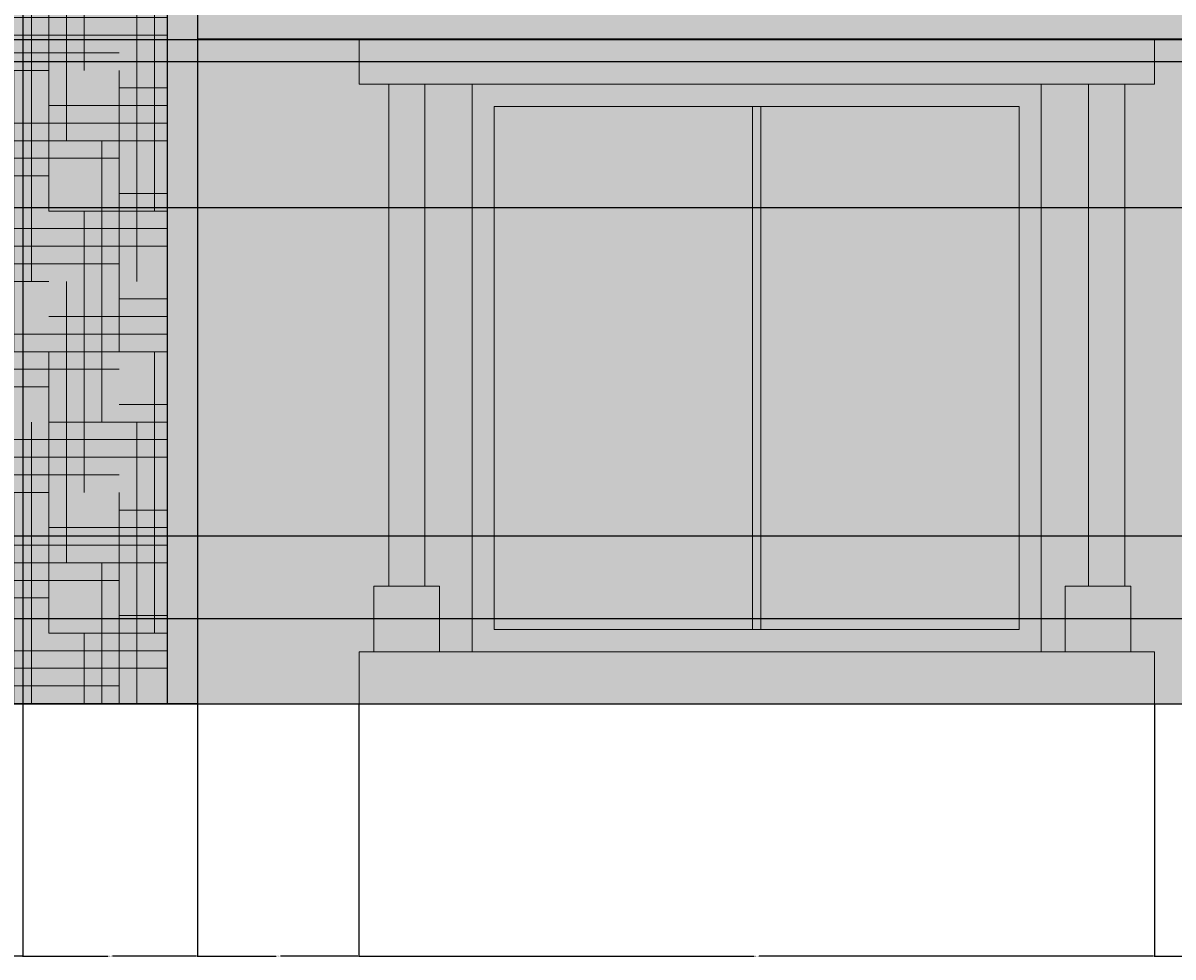
# Model space of a CAD drawing. Units: inches. Extents: x 3024 to 4744, y 1110 to 2100.
# Tile 14 of 29: x 3450 to 3657, y 1110 to 1279. Entities that reach past the tile are written whole.
import ezdxf

# ---------------------------------------------------------------- set-up
doc = ezdxf.new("R2010")
doc.units = ezdxf.units.IN
for name, color, linetype, lineweight in [('A-ANNO-DIMS', 2, 'Continuous', 18), ('A-ELEV', 7, 'Continuous', 25), ('A-ELEV-PATT', 252, 'Continuous', 13), ('A-GLAZ', 4, 'Continuous', 18)]:
    doc.layers.add(name, color=color, linetype=linetype, lineweight=lineweight)
doc.styles.get("Standard").update_dxf_attribs({"font": 'arial.ttf'})
doc.dimstyles.get("Standard").update_dxf_attribs({"dimtxt": 0.18, "dimasz": 0.18, "dimexe": 0.18, "dimexo": 0.0625, "dimgap": 0.09, "dimtad": 0, "dimtih": 1, "dimtoh": 1, "dimdec": 1, "dimzin": 0, "dimdsep": 46, "dimlunit": 3, "dimtxsty": 'Standard', "dimcen": 0.09, "dimadec": 0, "dimazin": 0, "dimtfac": 1, "dimtdec": 1, "dimtofl": 0, "dimtmove": 0, "dimatfit": 3, "dimfxl": 1, "dimtolj": 1, "dimtzin": 0, "dimarcsym": 0})

# ---------------------------------------------------------------- blocks, each defined once
blk = doc.blocks.new('WIN-BALCONY-A')
for p, q in [((3169.4, 1897.49), (3148.97, 1897.49)), ((3169.4, 1897.49), (3148.97, 1897.49)), ((3169.4, 1897.49), (3292.61, 1897.49)), ((3169.4, 1897.49), (3292.61, 1897.49)), ((3169.4, 1795.04), (3148.97, 1795.04)), ((3169.4, 1795.04), (3148.97, 1795.04)), ((3169.4, 1795.04), (3292.61, 1795.04)), ((3169.4, 1795.04), (3292.61, 1795.04))]:
    blk.add_line(p, q)
for points in [[(3148.97, 1897.49), (3148.97, 1905.61), (3292.61, 1905.61), (3292.61, 1897.49)], [(3148.97, 1897.49), (3148.97, 1905.61), (3292.61, 1905.61), (3292.61, 1897.49)], [(3292.61, 1795.04), (3292.61, 1785.61), (3148.97, 1785.61), (3148.97, 1795.04)], [(3292.61, 1795.04), (3292.61, 1785.61), (3148.97, 1785.61), (3148.97, 1795.04)]]:
    blk.add_lwpolyline(points)
for points in [[(3154.33, 1806.87), (3160.86, 1806.87), (3160.86, 1897.49), (3154.33, 1897.49)], [(3154.33, 1806.87), (3160.86, 1806.87), (3160.86, 1897.49), (3154.33, 1897.49)], [(3272.18, 1795.04), (3169.4, 1795.04), (3169.4, 1897.49), (3272.18, 1897.49)], [(3272.18, 1795.04), (3169.4, 1795.04), (3169.4, 1897.49), (3272.18, 1897.49)], [(3287.25, 1806.87), (3280.72, 1806.87), (3280.72, 1897.49), (3287.25, 1897.49)], [(3287.25, 1806.87), (3280.72, 1806.87), (3280.72, 1897.49), (3287.25, 1897.49)], [(3268.18, 1799.04), (3173.4, 1799.04), (3173.4, 1893.49), (3268.18, 1893.49)], [(3268.18, 1799.04), (3173.4, 1799.04), (3173.4, 1893.49), (3268.18, 1893.49)], [(3220.05, 1893.49), (3221.52, 1893.49), (3221.52, 1799.04), (3220.05, 1799.04)], [(3220.05, 1893.49), (3221.52, 1893.49), (3221.52, 1799.04), (3220.05, 1799.04)], [(3163.53, 1795.04), (3151.66, 1795.04), (3151.66, 1806.87), (3163.53, 1806.87)], [(3163.53, 1795.04), (3151.66, 1795.04), (3151.66, 1806.87), (3163.53, 1806.87)], [(3276.51, 1795.04), (3288.38, 1795.04), (3288.38, 1806.87), (3276.51, 1806.87)], [(3276.51, 1795.04), (3288.38, 1795.04), (3288.38, 1806.87), (3276.51, 1806.87)]]:
    blk.add_lwpolyline(points, close=True)
blk = doc.blocks.new('*D57')
at = {"layer": 'A-ANNO-DIMS', "color": 0, "lineweight": -2, "transparency": 16777216}
for p, q in [((3361.22, 1329.46), (3361.22, 1109.93)), ((3449.72, 1329.46), (3449.72, 1109.93)), ((3361.4, 1110.11), (3405.15, 1110.11)), ((3449.54, 1110.11), (3405.8, 1110.11))]:
    blk.add_line(p, q, dxfattribs=at)
at = {"layer": 'A-ANNO-DIMS', "color": 0, "transparency": 16777216}
for points in [[(3361.4, 1110.14), (3361.4, 1110.08), (3361.22, 1110.11)], [(3449.54, 1110.14), (3449.54, 1110.08), (3449.72, 1110.11)]]:
    blk.add_solid(points, dxfattribs=at)
at = {"layer": 'Defpoints', "color": 0, "transparency": 16777216}
for p in [(3361.22, 1329.52), (3449.72, 1329.52), (3449.72, 1110.11)]:
    blk.add_point(p, dxfattribs=at)
at = {"layer": 'A-ANNO-DIMS', "color": 0, "transparency": 16777216, "insert": (3405.47, 1110.11), "char_height": 0.18, "attachment_point": 5}
blk.add_mtext('\\A1;88.5', dxfattribs=at)
blk = doc.blocks.new('*D58')
at = {"layer": 'A-ANNO-DIMS', "color": 0, "lineweight": -2, "transparency": 16777216}
for p, q in [((3449.72, 1329.46), (3449.72, 1109.93)), ((3481.24, 1155.55), (3481.24, 1109.93)), ((3449.9, 1110.11), (3465.09, 1110.11)), ((3481.06, 1110.11), (3465.87, 1110.11))]:
    blk.add_line(p, q, dxfattribs=at)
at = {"layer": 'A-ANNO-DIMS', "color": 0, "transparency": 16777216}
for points in [[(3449.9, 1110.14), (3449.9, 1110.08), (3449.72, 1110.11)], [(3481.06, 1110.14), (3481.06, 1110.08), (3481.24, 1110.11)]]:
    blk.add_solid(points, dxfattribs=at)
at = {"layer": 'Defpoints', "color": 0, "transparency": 16777216}
for p in [(3449.72, 1329.52), (3481.24, 1155.61), (3481.24, 1110.11)]:
    blk.add_point(p, dxfattribs=at)
at = {"layer": 'A-ANNO-DIMS', "color": 0, "transparency": 16777216, "insert": (3465.48, 1110.11), "char_height": 0.18, "attachment_point": 5}
blk.add_mtext('\\A1;31.52', dxfattribs=at)
blk = doc.blocks.new('*D59')
at = {"layer": 'A-ANNO-DIMS', "color": 0, "lineweight": -2, "transparency": 16777216}
for p, q in [((3481.24, 1155.55), (3481.24, 1109.93)), ((3510.4, 1155.55), (3510.4, 1109.93)), ((3481.42, 1110.11), (3495.43, 1110.11)), ((3510.22, 1110.11), (3496.22, 1110.11))]:
    blk.add_line(p, q, dxfattribs=at)
at = {"layer": 'A-ANNO-DIMS', "color": 0, "transparency": 16777216}
for points in [[(3481.42, 1110.14), (3481.42, 1110.08), (3481.24, 1110.11)], [(3510.22, 1110.14), (3510.22, 1110.08), (3510.4, 1110.11)]]:
    blk.add_solid(points, dxfattribs=at)
at = {"layer": 'Defpoints', "color": 0, "transparency": 16777216}
for p in [(3481.24, 1155.61), (3510.4, 1155.61), (3510.4, 1110.11)]:
    blk.add_point(p, dxfattribs=at)
at = {"layer": 'A-ANNO-DIMS', "color": 0, "transparency": 16777216, "insert": (3495.82, 1110.11), "char_height": 0.18, "attachment_point": 5}
blk.add_mtext('\\A1;29.16', dxfattribs=at)
blk = doc.blocks.new('*D60')
at = {"layer": 'A-ANNO-DIMS', "color": 0, "lineweight": -2, "transparency": 16777216}
for p, q in [((3510.4, 1155.55), (3510.4, 1109.93)), ((3654.04, 1155.55), (3654.04, 1109.93)), ((3510.58, 1110.11), (3581.76, 1110.11)), ((3653.86, 1110.11), (3582.67, 1110.11))]:
    blk.add_line(p, q, dxfattribs=at)
at = {"layer": 'A-ANNO-DIMS', "color": 0, "transparency": 16777216}
for points in [[(3510.58, 1110.14), (3510.58, 1110.08), (3510.4, 1110.11)], [(3653.86, 1110.14), (3653.86, 1110.08), (3654.04, 1110.11)]]:
    blk.add_solid(points, dxfattribs=at)
at = {"layer": 'Defpoints', "color": 0, "transparency": 16777216}
for p in [(3510.4, 1155.61), (3654.04, 1155.61), (3654.04, 1110.11)]:
    blk.add_point(p, dxfattribs=at)
at = {"layer": 'A-ANNO-DIMS', "color": 0, "transparency": 16777216, "insert": (3582.22, 1110.11), "char_height": 0.18, "attachment_point": 5}
blk.add_mtext('\\A1;143.64', dxfattribs=at)
blk = doc.blocks.new('*D61')
at = {"layer": 'A-ANNO-DIMS', "color": 0, "lineweight": -2, "transparency": 16777216}
for p, q in [((3654.04, 1155.55), (3654.04, 1109.93)), ((3688.56, 1155.55), (3688.56, 1109.93)), ((3654.22, 1110.11), (3670.91, 1110.11)), ((3688.38, 1110.11), (3671.69, 1110.11))]:
    blk.add_line(p, q, dxfattribs=at)
at = {"layer": 'A-ANNO-DIMS', "color": 0, "transparency": 16777216}
for points in [[(3654.22, 1110.14), (3654.22, 1110.08), (3654.04, 1110.11)], [(3688.38, 1110.14), (3688.38, 1110.08), (3688.56, 1110.11)]]:
    blk.add_solid(points, dxfattribs=at)
at = {"layer": 'Defpoints', "color": 0, "transparency": 16777216}
for p in [(3654.04, 1155.61), (3688.56, 1155.61), (3688.56, 1110.11)]:
    blk.add_point(p, dxfattribs=at)
at = {"layer": 'A-ANNO-DIMS', "color": 0, "transparency": 16777216, "insert": (3671.3, 1110.11), "char_height": 0.18, "attachment_point": 5}
blk.add_mtext('\\A1;34.52', dxfattribs=at)
blk = doc.blocks.new('*D64')
at = {"layer": 'A-ANNO-DIMS', "color": 0, "lineweight": -2, "transparency": 16777216}
for p, q in [((3069.79, 1241.5), (3069.79, 2100.44)), ((3069.97, 2100.26), (3405.08, 2100.26)), ((3740.97, 2100.26), (3405.87, 2100.26)), ((3741.15, 1241.5), (3741.15, 2100.44))]:
    blk.add_line(p, q, dxfattribs=at)
at = {"layer": 'A-ANNO-DIMS', "color": 0, "transparency": 16777216}
for points in [[(3069.97, 2100.29), (3069.97, 2100.23), (3069.79, 2100.26)], [(3740.97, 2100.29), (3740.97, 2100.23), (3741.15, 2100.26)]]:
    blk.add_solid(points, dxfattribs=at)
at = {"layer": 'Defpoints', "color": 0, "transparency": 16777216}
for p in [(3741.15, 2100.26), (3069.79, 1241.43), (3741.15, 1241.43)]:
    blk.add_point(p, dxfattribs=at)
at = {"layer": 'A-ANNO-DIMS', "color": 0, "transparency": 16777216, "insert": (3405.47, 2100.26), "char_height": 0.18, "attachment_point": 5}
blk.add_mtext('\\A1;671.4', dxfattribs=at)
blk = doc.blocks.new('*D75')
at = {"layer": 'A-ANNO-DIMS', "color": 0, "lineweight": -2, "transparency": 16777216}
for p, q in [((3491.89, 2054.76), (3786.83, 2054.76)), ((3786.65, 2054.58), (3786.65, 1605.37)), ((3786.65, 1155.79), (3786.65, 1605)), ((3741.21, 1155.61), (3786.83, 1155.61))]:
    blk.add_line(p, q, dxfattribs=at)
at = {"layer": 'A-ANNO-DIMS', "color": 0, "transparency": 16777216}
for points in [[(3786.62, 2054.58), (3786.68, 2054.58), (3786.65, 2054.76)], [(3786.62, 1155.79), (3786.68, 1155.79), (3786.65, 1155.61)]]:
    blk.add_solid(points, dxfattribs=at)
at = {"layer": 'Defpoints', "color": 0, "transparency": 16777216}
for p in [(3491.83, 2054.76), (3786.65, 2054.76), (3741.15, 1155.61)]:
    blk.add_point(p, dxfattribs=at)
at = {"layer": 'A-ANNO-DIMS', "color": 0, "transparency": 16777216, "insert": (3786.65, 1605.18), "char_height": 0.18, "attachment_point": 5}
blk.add_mtext('\\A1;899.1', dxfattribs=at)
blk = doc.blocks.new('*D120')
at = {"layer": 'A-ANNO-DIMS', "color": 0, "lineweight": -2, "transparency": 16777216}
for p, q in [((3270.45, 1271.61), (3786.83, 1271.61)), ((3786.65, 1271.43), (3786.65, 1221.5)), ((3786.65, 1171.2), (3786.65, 1221.14)), ((3274.45, 1171.02), (3786.83, 1171.02))]:
    blk.add_line(p, q, dxfattribs=at)
at = {"layer": 'A-ANNO-DIMS', "color": 0, "transparency": 16777216}
for points in [[(3786.62, 1271.43), (3786.68, 1271.43), (3786.65, 1271.61)], [(3786.62, 1171.2), (3786.68, 1171.2), (3786.65, 1171.02)]]:
    blk.add_solid(points, dxfattribs=at)
at = {"layer": 'Defpoints', "color": 0, "transparency": 16777216}
for p in [(3270.39, 1271.61), (3786.65, 1271.61), (3274.39, 1171.02)]:
    blk.add_point(p, dxfattribs=at)
at = {"layer": 'A-ANNO-DIMS', "color": 0, "transparency": 16777216, "insert": (3786.65, 1221.32), "char_height": 0.18, "attachment_point": 5}
blk.add_mtext('\\A1;100.59', dxfattribs=at)
blk = doc.blocks.new('*D121')
at = {"layer": 'A-ANNO-DIMS', "color": 0, "lineweight": -2, "transparency": 16777216}
for p, q in [((3274.45, 1275.61), (3786.83, 1275.61)), ((3786.65, 1275.43), (3786.65, 1273.79)), ((3786.65, 1271.79), (3786.65, 1273.43)), ((3270.45, 1271.61), (3786.83, 1271.61))]:
    blk.add_line(p, q, dxfattribs=at)
at = {"layer": 'A-ANNO-DIMS', "color": 0, "transparency": 16777216}
for points in [[(3786.62, 1275.43), (3786.68, 1275.43), (3786.65, 1275.61)], [(3786.62, 1271.79), (3786.68, 1271.79), (3786.65, 1271.61)]]:
    blk.add_solid(points, dxfattribs=at)
at = {"layer": 'Defpoints', "color": 0, "transparency": 16777216}
for p in [(3274.39, 1275.61), (3786.65, 1275.61), (3270.39, 1271.61)]:
    blk.add_point(p, dxfattribs=at)
at = {"layer": 'A-ANNO-DIMS', "color": 0, "transparency": 16777216, "insert": (3786.65, 1273.61), "char_height": 0.18, "attachment_point": 5}
blk.add_mtext('\\A1;4.00', dxfattribs=at)
blk = doc.blocks.new('*D122')
at = {"layer": 'A-ANNO-DIMS', "color": 0, "lineweight": -2, "transparency": 16777216}
for p, q in [((3228.45, 1185.95), (3786.83, 1185.95)), ((3786.65, 1185.77), (3786.65, 1178.67)), ((3786.65, 1171.2), (3786.65, 1178.31)), ((3270.45, 1171.02), (3786.83, 1171.02))]:
    blk.add_line(p, q, dxfattribs=at)
at = {"layer": 'A-ANNO-DIMS', "color": 0, "transparency": 16777216}
for points in [[(3786.62, 1185.77), (3786.68, 1185.77), (3786.65, 1185.95)], [(3786.62, 1171.2), (3786.68, 1171.2), (3786.65, 1171.02)]]:
    blk.add_solid(points, dxfattribs=at)
at = {"layer": 'Defpoints', "color": 0, "transparency": 16777216}
for p in [(3228.39, 1185.95), (3270.39, 1171.02), (3786.65, 1171.02)]:
    blk.add_point(p, dxfattribs=at)
at = {"layer": 'A-ANNO-DIMS', "color": 0, "transparency": 16777216, "insert": (3786.65, 1178.49), "char_height": 0.18, "attachment_point": 5}
blk.add_mtext('\\A1;14.928', dxfattribs=at)
blk = doc.blocks.new('*D123')
at = {"layer": 'A-ANNO-DIMS', "color": 0, "lineweight": -2, "transparency": 16777216}
for p, q in [((3228.45, 1245.27), (3786.83, 1245.27)), ((3786.65, 1245.09), (3786.65, 1215.79)), ((3786.65, 1186.13), (3786.65, 1215.43)), ((3228.45, 1185.95), (3786.83, 1185.95))]:
    blk.add_line(p, q, dxfattribs=at)
at = {"layer": 'A-ANNO-DIMS', "color": 0, "transparency": 16777216}
for points in [[(3786.62, 1245.09), (3786.68, 1245.09), (3786.65, 1245.27)], [(3786.62, 1186.13), (3786.68, 1186.13), (3786.65, 1185.95)]]:
    blk.add_solid(points, dxfattribs=at)
at = {"layer": 'Defpoints', "color": 0, "transparency": 16777216}
for p in [(3228.39, 1245.27), (3786.65, 1245.27), (3228.39, 1185.95)]:
    blk.add_point(p, dxfattribs=at)
at = {"layer": 'A-ANNO-DIMS', "color": 0, "transparency": 16777216, "insert": (3786.65, 1215.61), "char_height": 0.18, "attachment_point": 5}
blk.add_mtext('\\A1;59.32', dxfattribs=at)

msp = doc.modelspace()

# ---------------------------------------------------------------- hatches: boundary and pattern name
at = {"layer": 'A-ELEV-PATT'}
h = msp.add_hatch(color=256, dxfattribs=at)
h.dxf.hatch_style = 1
h.paths.add_polyline_path([(3491.8271, 2054.7584), (3320.5658, 2054.7584), (3320.5658, 2043.5286), (3491.8271, 2043.5286)])
h.paths.add_polyline_path([(3292.6051, 1905.6112), (3148.9694, 1905.6112), (3148.9694, 1897.4879), (3169.3964, 1897.4879), (3292.6051, 1897.4879)])
h.paths.add_polyline_path([(3292.6051, 1795.0431), (3169.3964, 1795.0431), (3148.9694, 1795.0431), (3148.9694, 1785.6112), (3292.6051, 1785.6112)])
h.paths.add_polyline_path([(3292.6051, 1779.6112), (3148.9694, 1779.6112), (3148.9694, 1771.4879), (3169.3964, 1771.4879), (3292.6051, 1771.4879)])
h.paths.add_polyline_path([(3292.6051, 1669.0431), (3169.3964, 1669.0431), (3148.9694, 1669.0431), (3148.9694, 1659.6112), (3292.6051, 1659.6112)])
h.paths.add_polyline_path([(3292.6051, 1653.6112), (3148.9694, 1653.6112), (3148.9694, 1645.4879), (3169.3964, 1645.4879), (3292.6051, 1645.4879)])
h.paths.add_polyline_path([(3292.6051, 1543.0431), (3169.3964, 1543.0431), (3148.9694, 1543.0431), (3148.9694, 1533.6112), (3292.6051, 1533.6112)])
h.paths.add_polyline_path([(3292.6051, 1527.6112), (3148.9694, 1527.6112), (3148.9694, 1519.4879), (3169.3964, 1519.4879), (3292.6051, 1519.4879)])
h.paths.add_polyline_path([(3292.6051, 1401.6112), (3148.9694, 1401.6112), (3148.9694, 1393.4879), (3169.3964, 1393.4879), (3292.6051, 1393.4879)])
h.paths.add_polyline_path([(3292.6051, 1417.0431), (3169.3964, 1417.0431), (3148.9694, 1417.0431), (3148.9694, 1407.6112), (3292.6051, 1407.6112)])
h.paths.add_polyline_path([(3292.6051, 1291.0431), (3169.3964, 1291.0431), (3148.9694, 1291.0431), (3148.9694, 1281.6112), (3292.6051, 1281.6112)])
h.paths.add_polyline_path([(3654.037, 1165.0431), (3530.8283, 1165.0431), (3510.4013, 1165.0431), (3510.4013, 1155.6112), (3654.037, 1155.6112)])
h.paths.add_polyline_path([(3654.037, 1275.6112), (3510.4013, 1275.6112), (3510.4013, 1267.4879), (3530.8283, 1267.4879), (3654.037, 1267.4879)])
h.paths.add_polyline_path([(3654.037, 1291.0431), (3530.8283, 1291.0431), (3510.4013, 1291.0431), (3510.4013, 1281.6112), (3654.037, 1281.6112)])
h.paths.add_polyline_path([(3654.037, 1417.0431), (3530.8283, 1417.0431), (3510.4013, 1417.0431), (3510.4013, 1407.6112), (3654.037, 1407.6112)])
h.paths.add_polyline_path([(3654.037, 1401.6112), (3510.4013, 1401.6112), (3510.4013, 1393.4879), (3530.8283, 1393.4879), (3654.037, 1393.4879)])
h.paths.add_polyline_path([(3654.037, 1543.0431), (3530.8283, 1543.0431), (3510.4013, 1543.0431), (3510.4013, 1533.6112), (3654.037, 1533.6112)])
h.paths.add_polyline_path([(3654.037, 1527.6112), (3510.4013, 1527.6112), (3510.4013, 1519.4879), (3530.8283, 1519.4879), (3654.037, 1519.4879)])
h.paths.add_polyline_path([(3654.037, 1653.6112), (3510.4013, 1653.6112), (3510.4013, 1645.4879), (3530.8283, 1645.4879), (3654.037, 1645.4879)])
h.paths.add_polyline_path([(3654.037, 1669.0431), (3530.8283, 1669.0431), (3510.4013, 1669.0431), (3510.4013, 1659.6112), (3654.037, 1659.6112)])
h.paths.add_polyline_path([(3654.037, 1779.6112), (3510.4013, 1779.6112), (3510.4013, 1771.4879), (3530.8283, 1771.4879), (3654.037, 1771.4879)])
h.paths.add_polyline_path([(3654.037, 1795.0431), (3530.8283, 1795.0431), (3510.4013, 1795.0431), (3510.4013, 1785.6112), (3654.037, 1785.6112)])
h.paths.add_polyline_path([(3654.037, 1905.6112), (3510.4013, 1905.6112), (3510.4013, 1897.4879), (3530.8283, 1897.4879), (3654.037, 1897.4879)])
h = msp.add_hatch(color=256, dxfattribs=at)
h.dxf.hatch_style = 1
h.paths.add_polyline_path([(3335.1044, 2043.5286), (3329.7033, 2043.5286), (3329.7033, 1155.6112), (3335.1044, 1155.6112)])
h.paths.add_polyline_path([(3481.2411, 2043.5286), (3335.1044, 2043.5286), (3335.1044, 1155.6112), (3481.2411, 1155.6112)])
h.paths.add_polyline_path([(3449.7202, 1329.5246), (3361.2242, 1329.5246), (3361.2242, 1436.6064), (3449.7202, 1436.6064)], flags=16)
h.paths.add_polyline_path([(3445.7202, 1333.5246), (3365.2242, 1333.5246), (3365.2242, 1432.6064), (3445.7202, 1432.6064)], flags=0)
h.paths.add_polyline_path([(3449.7202, 1455.5246), (3361.2242, 1455.5246), (3361.2242, 1562.6064), (3449.7202, 1562.6064)], flags=16)
h.paths.add_polyline_path([(3445.7202, 1459.5246), (3365.2242, 1459.5246), (3365.2242, 1558.6064), (3445.7202, 1558.6064)], flags=0)
h.paths.add_polyline_path([(3449.7202, 1581.5246), (3361.2242, 1581.5246), (3361.2242, 1688.6064), (3449.7202, 1688.6064)], flags=16)
h.paths.add_polyline_path([(3445.7202, 1585.5246), (3365.2242, 1585.5246), (3365.2242, 1684.6064), (3445.7202, 1684.6064)], flags=0)
h.paths.add_polyline_path([(3449.7202, 1707.5246), (3361.2242, 1707.5246), (3361.2242, 1814.6064), (3449.7202, 1814.6064)], flags=16)
h.paths.add_polyline_path([(3445.7202, 1711.5246), (3365.2242, 1711.5246), (3365.2242, 1810.6064), (3445.7202, 1810.6064)], flags=0)
h.paths.add_polyline_path([(3449.7202, 1833.5246), (3361.2242, 1833.5246), (3361.2242, 1940.6064), (3449.7202, 1940.6064)], flags=16)
h.paths.add_polyline_path([(3445.7202, 1837.5246), (3365.2242, 1837.5246), (3365.2242, 1936.6064), (3445.7202, 1936.6064)], flags=0)
h = msp.add_hatch(color=256, dxfattribs=at)
h.dxf.hatch_style = 1
h.paths.add_polyline_path([(3475.84, 2043.5286), (3335.1044, 2043.5286), (3335.1044, 1155.6112), (3475.84, 1155.6112)])
h.paths.add_polyline_path([(3449.7202, 1940.6064), (3449.7202, 1833.5246), (3361.2242, 1833.5246), (3361.2242, 1940.6064)], flags=16)
h.paths.add_polyline_path([(3445.7202, 1936.6064), (3445.7202, 1837.5246), (3365.2242, 1837.5246), (3365.2242, 1936.6064)], flags=0)
h.paths.add_polyline_path([(3449.7202, 1814.6064), (3449.7202, 1707.5246), (3361.2242, 1707.5246), (3361.2242, 1814.6064)], flags=16)
h.paths.add_polyline_path([(3445.7202, 1810.6064), (3445.7202, 1711.5246), (3365.2242, 1711.5246), (3365.2242, 1810.6064)], flags=0)
h.paths.add_polyline_path([(3449.7202, 1688.6064), (3449.7202, 1581.5246), (3361.2242, 1581.5246), (3361.2242, 1688.6064)], flags=16)
h.paths.add_polyline_path([(3445.7202, 1684.6064), (3445.7202, 1585.5246), (3365.2242, 1585.5246), (3365.2242, 1684.6064)], flags=0)
h.paths.add_polyline_path([(3449.7202, 1562.6064), (3449.7202, 1455.5246), (3361.2242, 1455.5246), (3361.2242, 1562.6064)], flags=16)
h.paths.add_polyline_path([(3445.7202, 1558.6064), (3445.7202, 1459.5246), (3365.2242, 1459.5246), (3365.2242, 1558.6064)], flags=0)
h.paths.add_polyline_path([(3449.7202, 1436.6064), (3449.7202, 1329.5246), (3361.2242, 1329.5246), (3361.2242, 1436.6064)], flags=16)
h.paths.add_polyline_path([(3445.7202, 1432.6064), (3445.7202, 1333.5246), (3365.2242, 1333.5246), (3365.2242, 1432.6064)], flags=0)
h = msp.add_hatch(dxfattribs=at)
h.set_pattern_fill('HOUND', color=256, scale=2)
h.paths.add_polyline_path([(3475.84, 2043.5286), (3335.1044, 2043.5286), (3335.1044, 1155.6112), (3475.84, 1155.6112)])
h.paths.add_polyline_path([(3449.7202, 1940.6064), (3449.7202, 1833.5246), (3361.2242, 1833.5246), (3361.2242, 1940.6064)], flags=16)
h.paths.add_polyline_path([(3445.7202, 1936.6064), (3445.7202, 1837.5246), (3365.2242, 1837.5246), (3365.2242, 1936.6064)], flags=0)
h.paths.add_polyline_path([(3449.7202, 1814.6064), (3449.7202, 1707.5246), (3361.2242, 1707.5246), (3361.2242, 1814.6064)], flags=16)
h.paths.add_polyline_path([(3445.7202, 1810.6064), (3445.7202, 1711.5246), (3365.2242, 1711.5246), (3365.2242, 1810.6064)], flags=0)
h.paths.add_polyline_path([(3449.7202, 1688.6064), (3449.7202, 1581.5246), (3361.2242, 1581.5246), (3361.2242, 1688.6064)], flags=16)
h.paths.add_polyline_path([(3445.7202, 1684.6064), (3445.7202, 1585.5246), (3365.2242, 1585.5246), (3365.2242, 1684.6064)], flags=0)
h.paths.add_polyline_path([(3449.7202, 1562.6064), (3449.7202, 1455.5246), (3361.2242, 1455.5246), (3361.2242, 1562.6064)], flags=16)
h.paths.add_polyline_path([(3445.7202, 1558.6064), (3445.7202, 1459.5246), (3365.2242, 1459.5246), (3365.2242, 1558.6064)], flags=0)
h.paths.add_polyline_path([(3449.7202, 1436.6064), (3449.7202, 1329.5246), (3361.2242, 1329.5246), (3361.2242, 1436.6064)], flags=16)
h.paths.add_polyline_path([(3445.7202, 1432.6064), (3445.7202, 1333.5246), (3365.2242, 1333.5246), (3365.2242, 1432.6064)], flags=0)
h = msp.add_hatch(color=256, dxfattribs=at)
h.dxf.hatch_style = 1
h.paths.add_polyline_path([(3154.3287, 1897.4879), (3148.9694, 1897.4879), (3148.9694, 1905.6112), (3105.4722, 1905.6112), (3105.4722, 1785.6112), (3148.9694, 1785.6112), (3148.9694, 1795.0431), (3151.6604, 1795.0431), (3151.6604, 1806.8674), (3154.3287, 1806.8674)])
h.paths.add_polyline_path([(3329.7033, 1905.6112), (3292.6051, 1905.6112), (3292.6051, 1897.4879), (3287.2458, 1897.4879), (3287.2458, 1806.8674), (3288.3759, 1806.8674), (3288.3759, 1795.0431), (3292.6051, 1795.0431), (3292.6051, 1785.6112), (3329.7033, 1785.6112)])
h.paths.add_polyline_path([(3154.3287, 1771.4879), (3148.9694, 1771.4879), (3148.9694, 1779.6112), (3105.4722, 1779.6112), (3105.4722, 1659.6112), (3148.9694, 1659.6112), (3148.9694, 1669.0431), (3151.6604, 1669.0431), (3151.6604, 1680.8674), (3154.3287, 1680.8674)])
h.paths.add_polyline_path([(3329.7033, 1779.6112), (3292.6051, 1779.6112), (3292.6051, 1771.4879), (3287.2458, 1771.4879), (3287.2458, 1680.8674), (3288.3759, 1680.8674), (3288.3759, 1669.0431), (3292.6051, 1669.0431), (3292.6051, 1659.6112), (3329.7033, 1659.6112)])
h.paths.add_polyline_path([(3154.3287, 1645.4879), (3148.9694, 1645.4879), (3148.9694, 1653.6112), (3105.4722, 1653.6112), (3105.4722, 1533.6112), (3148.9694, 1533.6112), (3148.9694, 1543.0431), (3151.6604, 1543.0431), (3151.6604, 1554.8674), (3154.3287, 1554.8674)])
h.paths.add_polyline_path([(3329.7033, 1653.6112), (3292.6051, 1653.6112), (3292.6051, 1645.4879), (3287.2458, 1645.4879), (3287.2458, 1554.8674), (3288.3759, 1554.8674), (3288.3759, 1543.0431), (3292.6051, 1543.0431), (3292.6051, 1533.6112), (3329.7033, 1533.6112)])
h.paths.add_polyline_path([(3329.7033, 1527.6112), (3292.6051, 1527.6112), (3292.6051, 1519.4879), (3287.2458, 1519.4879), (3287.2458, 1428.8674), (3288.3759, 1428.8674), (3288.3759, 1417.0431), (3292.6051, 1417.0431), (3292.6051, 1407.6112), (3329.7033, 1407.6112)])
h.paths.add_polyline_path([(3329.7033, 1401.6112), (3292.6051, 1401.6112), (3292.6051, 1393.4879), (3287.2458, 1393.4879), (3287.2458, 1302.8674), (3288.3759, 1302.8674), (3288.3759, 1291.0431), (3292.6051, 1291.0431), (3292.6051, 1281.6112), (3329.7033, 1281.6112)])
h.paths.add_polyline_path([(3154.3287, 1393.4879), (3148.9694, 1393.4879), (3148.9694, 1401.6112), (3105.4722, 1401.6112), (3105.4722, 1281.6112), (3148.9694, 1281.6112), (3148.9694, 1291.0431), (3151.6604, 1291.0431), (3151.6604, 1302.8674), (3154.3287, 1302.8674)])
h.paths.add_polyline_path([(3154.3287, 1519.4879), (3148.9694, 1519.4879), (3148.9694, 1527.6112), (3105.4722, 1527.6112), (3105.4722, 1407.6112), (3148.9694, 1407.6112), (3148.9694, 1417.0431), (3151.6604, 1417.0431), (3151.6604, 1428.8674), (3154.3287, 1428.8674)])
h.paths.add_polyline_path([(3515.7606, 1897.4879), (3510.4013, 1897.4879), (3510.4013, 1905.6112), (3481.2411, 1905.6112), (3481.2411, 1785.6112), (3510.4013, 1785.6112), (3510.4013, 1795.0431), (3513.0923, 1795.0431), (3513.0923, 1806.8674), (3515.7606, 1806.8674)])
h.paths.add_polyline_path([(3688.5588, 1905.6112), (3654.037, 1905.6112), (3654.037, 1897.4879), (3648.6777, 1897.4879), (3648.6777, 1806.8674), (3649.8078, 1806.8674), (3649.8078, 1795.0431), (3654.037, 1795.0431), (3654.037, 1785.6112), (3688.5588, 1785.6112)])
h.paths.add_polyline_path([(3515.7606, 1771.4879), (3510.4013, 1771.4879), (3510.4013, 1779.6112), (3481.2411, 1779.6112), (3481.2411, 1659.6112), (3510.4013, 1659.6112), (3510.4013, 1669.0431), (3513.0923, 1669.0431), (3513.0923, 1680.8674), (3515.7606, 1680.8674)])
h.paths.add_polyline_path([(3688.5588, 1779.6112), (3654.037, 1779.6112), (3654.037, 1771.4879), (3648.6777, 1771.4879), (3648.6777, 1680.8674), (3649.8078, 1680.8674), (3649.8078, 1669.0431), (3654.037, 1669.0431), (3654.037, 1659.6112), (3688.5588, 1659.6112)])
h.paths.add_polyline_path([(3515.7606, 1645.4879), (3510.4013, 1645.4879), (3510.4013, 1653.6112), (3481.2411, 1653.6112), (3481.2411, 1533.6112), (3510.4013, 1533.6112), (3510.4013, 1543.0431), (3513.0923, 1543.0431), (3513.0923, 1554.8674), (3515.7606, 1554.8674)])
h.paths.add_polyline_path([(3688.5588, 1653.6112), (3654.037, 1653.6112), (3654.037, 1645.4879), (3648.6777, 1645.4879), (3648.6777, 1554.8674), (3649.8078, 1554.8674), (3649.8078, 1543.0431), (3654.037, 1543.0431), (3654.037, 1533.6112), (3688.5588, 1533.6112)])
h.paths.add_polyline_path([(3515.7606, 1519.4879), (3510.4013, 1519.4879), (3510.4013, 1527.6112), (3481.2411, 1527.6112), (3481.2411, 1407.6112), (3510.4013, 1407.6112), (3510.4013, 1417.0431), (3513.0923, 1417.0431), (3513.0923, 1428.8674), (3515.7606, 1428.8674)])
h.paths.add_polyline_path([(3688.5588, 1527.6112), (3654.037, 1527.6112), (3654.037, 1519.4879), (3648.6777, 1519.4879), (3648.6777, 1428.8674), (3649.8078, 1428.8674), (3649.8078, 1417.0431), (3654.037, 1417.0431), (3654.037, 1407.6112), (3688.5588, 1407.6112)])
h.paths.add_polyline_path([(3515.7606, 1393.4879), (3510.4013, 1393.4879), (3510.4013, 1401.6112), (3481.2411, 1401.6112), (3481.2411, 1281.6112), (3510.4013, 1281.6112), (3510.4013, 1291.0431), (3513.0923, 1291.0431), (3513.0923, 1302.8674), (3515.7606, 1302.8674)])
h.paths.add_polyline_path([(3688.5588, 1401.6112), (3654.037, 1401.6112), (3654.037, 1393.4879), (3648.6777, 1393.4879), (3648.6777, 1302.8674), (3649.8078, 1302.8674), (3649.8078, 1291.0431), (3654.037, 1291.0431), (3654.037, 1281.6112), (3688.5588, 1281.6112)])
h.paths.add_polyline_path([(3515.7606, 1267.4879), (3510.4013, 1267.4879), (3510.4013, 1275.6112), (3481.2411, 1275.6112), (3481.2411, 1155.6112), (3510.4013, 1155.6112), (3510.4013, 1165.0431), (3513.0923, 1165.0431), (3513.0923, 1176.8674), (3515.7606, 1176.8674)])
h.paths.add_polyline_path([(3688.5588, 1275.6112), (3654.037, 1275.6112), (3654.037, 1267.4879), (3648.6777, 1267.4879), (3648.6777, 1176.8674), (3649.8078, 1176.8674), (3649.8078, 1165.0431), (3654.037, 1165.0431), (3654.037, 1155.6112), (3688.5588, 1155.6112)])
h.paths.add_polyline_path([(3112.3838, 1275.6112), (3105.4722, 1275.6112), (3105.4722, 1171.0239), (3112.3838, 1171.0239)])
h = msp.add_hatch(color=256, dxfattribs=at)
h.dxf.hatch_style = 1
h.paths.add_polyline_path([(3160.8586, 1897.4879), (3154.3287, 1897.4879), (3154.3287, 1806.8674), (3160.8586, 1806.8674)])
h.paths.add_polyline_path([(3287.2458, 1897.4879), (3280.716, 1897.4879), (3280.716, 1806.8674), (3287.2458, 1806.8674)])
h.paths.add_polyline_path([(3160.8586, 1771.4879), (3154.3287, 1771.4879), (3154.3287, 1680.8674), (3160.8586, 1680.8674)])
h.paths.add_polyline_path([(3287.2458, 1771.4879), (3280.716, 1771.4879), (3280.716, 1680.8674), (3287.2458, 1680.8674)])
h.paths.add_polyline_path([(3160.8586, 1645.4879), (3154.3287, 1645.4879), (3154.3287, 1554.8674), (3160.8586, 1554.8674)])
h.paths.add_polyline_path([(3287.2458, 1645.4879), (3280.716, 1645.4879), (3280.716, 1554.8674), (3287.2458, 1554.8674)])
h.paths.add_polyline_path([(3160.8586, 1519.4879), (3154.3287, 1519.4879), (3154.3287, 1428.8674), (3160.8586, 1428.8674)])
h.paths.add_polyline_path([(3287.2458, 1519.4879), (3280.716, 1519.4879), (3280.716, 1428.8674), (3287.2458, 1428.8674)])
h.paths.add_polyline_path([(3160.8586, 1393.4879), (3154.3287, 1393.4879), (3154.3287, 1302.8674), (3160.8586, 1302.8674)])
h.paths.add_polyline_path([(3287.2458, 1393.4879), (3280.716, 1393.4879), (3280.716, 1302.8674), (3287.2458, 1302.8674)])
h.paths.add_polyline_path([(3648.6777, 1267.4879), (3642.1479, 1267.4879), (3642.1479, 1176.8674), (3648.6777, 1176.8674)])
h.paths.add_polyline_path([(3522.2905, 1267.4879), (3515.7606, 1267.4879), (3515.7606, 1176.8674), (3522.2905, 1176.8674)])
h.paths.add_polyline_path([(3522.2905, 1393.4879), (3515.7606, 1393.4879), (3515.7606, 1302.8674), (3522.2905, 1302.8674)])
h.paths.add_polyline_path([(3648.6777, 1393.4879), (3642.1479, 1393.4879), (3642.1479, 1302.8674), (3648.6777, 1302.8674)])
h.paths.add_polyline_path([(3522.2905, 1519.4879), (3515.7606, 1519.4879), (3515.7606, 1428.8674), (3522.2905, 1428.8674)])
h.paths.add_polyline_path([(3648.6777, 1519.4879), (3642.1479, 1519.4879), (3642.1479, 1428.8674), (3648.6777, 1428.8674)])
h.paths.add_polyline_path([(3522.2905, 1645.4879), (3515.7606, 1645.4879), (3515.7606, 1554.8674), (3522.2905, 1554.8674)])
h.paths.add_polyline_path([(3522.2905, 1771.4879), (3515.7606, 1771.4879), (3515.7606, 1680.8674), (3522.2905, 1680.8674)])
h.paths.add_polyline_path([(3648.6777, 1645.4879), (3642.1479, 1645.4879), (3642.1479, 1554.8674), (3648.6777, 1554.8674)])
h.paths.add_polyline_path([(3648.6777, 1771.4879), (3642.1479, 1771.4879), (3642.1479, 1680.8674), (3648.6777, 1680.8674)])
h.paths.add_polyline_path([(3648.6777, 1897.4879), (3642.1479, 1897.4879), (3642.1479, 1806.8674), (3648.6777, 1806.8674)])
h.paths.add_polyline_path([(3522.2905, 1897.4879), (3515.7606, 1897.4879), (3515.7606, 1806.8674), (3522.2905, 1806.8674)])
h = msp.add_hatch(color=256, dxfattribs=at)
h.dxf.hatch_style = 1
h.paths.add_polyline_path([(3169.3964, 1897.4879), (3160.8586, 1897.4879), (3160.8586, 1806.8674), (3163.5269, 1806.8674), (3163.5269, 1795.0431), (3169.3964, 1795.0431)])
h.paths.add_polyline_path([(3280.716, 1897.4879), (3272.1781, 1897.4879), (3272.1781, 1795.0431), (3276.5094, 1795.0431), (3276.5094, 1806.8674), (3280.716, 1806.8674)])
h.paths.add_polyline_path([(3280.716, 1771.4879), (3272.1781, 1771.4879), (3272.1781, 1669.0431), (3276.5094, 1669.0431), (3276.5094, 1680.8674), (3280.716, 1680.8674)])
h.paths.add_polyline_path([(3169.3964, 1771.4879), (3160.8586, 1771.4879), (3160.8586, 1680.8674), (3163.5269, 1680.8674), (3163.5269, 1669.0431), (3169.3964, 1669.0431)])
h.paths.add_polyline_path([(3169.3964, 1645.4879), (3160.8586, 1645.4879), (3160.8586, 1554.8674), (3163.5269, 1554.8674), (3163.5269, 1543.0431), (3169.3964, 1543.0431)])
h.paths.add_polyline_path([(3280.716, 1645.4879), (3272.1781, 1645.4879), (3272.1781, 1543.0431), (3276.5094, 1543.0431), (3276.5094, 1554.8674), (3280.716, 1554.8674)])
h.paths.add_polyline_path([(3169.3964, 1519.4879), (3160.8586, 1519.4879), (3160.8586, 1428.8674), (3163.5269, 1428.8674), (3163.5269, 1417.0431), (3169.3964, 1417.0431)])
h.paths.add_polyline_path([(3280.716, 1519.4879), (3272.1781, 1519.4879), (3272.1781, 1417.0431), (3276.5094, 1417.0431), (3276.5094, 1428.8674), (3280.716, 1428.8674)])
h.paths.add_polyline_path([(3169.3964, 1393.4879), (3160.8586, 1393.4879), (3160.8586, 1302.8674), (3163.5269, 1302.8674), (3163.5269, 1291.0431), (3169.3964, 1291.0431)])
h.paths.add_polyline_path([(3280.716, 1393.4879), (3272.1781, 1393.4879), (3272.1781, 1291.0431), (3276.5094, 1291.0431), (3276.5094, 1302.8674), (3280.716, 1302.8674)])
h.paths.add_polyline_path([(3642.1479, 1267.4879), (3633.61, 1267.4879), (3633.61, 1165.0431), (3637.9413, 1165.0431), (3637.9413, 1176.8674), (3642.1479, 1176.8674)])
h.paths.add_polyline_path([(3530.8283, 1267.4879), (3522.2905, 1267.4879), (3522.2905, 1176.8674), (3524.9588, 1176.8674), (3524.9588, 1165.0431), (3530.8283, 1165.0431)])
h.paths.add_polyline_path([(3642.1479, 1393.4879), (3633.61, 1393.4879), (3633.61, 1291.0431), (3637.9413, 1291.0431), (3637.9413, 1302.8674), (3642.1479, 1302.8674)])
h.paths.add_polyline_path([(3530.8283, 1393.4879), (3522.2905, 1393.4879), (3522.2905, 1302.8674), (3524.9588, 1302.8674), (3524.9588, 1291.0431), (3530.8283, 1291.0431)])
h.paths.add_polyline_path([(3530.8283, 1519.4879), (3522.2905, 1519.4879), (3522.2905, 1428.8674), (3524.9588, 1428.8674), (3524.9588, 1417.0431), (3530.8283, 1417.0431)])
h.paths.add_polyline_path([(3642.1479, 1519.4879), (3633.61, 1519.4879), (3633.61, 1417.0431), (3637.9413, 1417.0431), (3637.9413, 1428.8674), (3642.1479, 1428.8674)])
h.paths.add_polyline_path([(3530.8283, 1645.4879), (3522.2905, 1645.4879), (3522.2905, 1554.8674), (3524.9588, 1554.8674), (3524.9588, 1543.0431), (3530.8283, 1543.0431)])
h.paths.add_polyline_path([(3642.1479, 1645.4879), (3633.61, 1645.4879), (3633.61, 1543.0431), (3637.9413, 1543.0431), (3637.9413, 1554.8674), (3642.1479, 1554.8674)])
h.paths.add_polyline_path([(3642.1479, 1771.4879), (3633.61, 1771.4879), (3633.61, 1669.0431), (3637.9413, 1669.0431), (3637.9413, 1680.8674), (3642.1479, 1680.8674)])
h.paths.add_polyline_path([(3530.8283, 1771.4879), (3522.2905, 1771.4879), (3522.2905, 1680.8674), (3524.9588, 1680.8674), (3524.9588, 1669.0431), (3530.8283, 1669.0431)])
h.paths.add_polyline_path([(3530.8283, 1897.4879), (3522.2905, 1897.4879), (3522.2905, 1806.8674), (3524.9588, 1806.8674), (3524.9588, 1795.0431), (3530.8283, 1795.0431)])
h.paths.add_polyline_path([(3642.1479, 1897.4879), (3633.61, 1897.4879), (3633.61, 1795.0431), (3637.9413, 1795.0431), (3637.9413, 1806.8674), (3642.1479, 1806.8674)])
h = msp.add_hatch(color=256, dxfattribs=at)
h.dxf.hatch_style = 1
h.paths.add_polyline_path([(3220.0505, 1893.4879), (3173.3964, 1893.4879), (3173.3964, 1799.0431), (3220.0505, 1799.0431)])
h.paths.add_polyline_path([(3268.1781, 1893.4879), (3221.5241, 1893.4879), (3221.5241, 1799.0431), (3268.1781, 1799.0431)])
h.paths.add_polyline_path([(3581.4824, 1893.4879), (3534.8283, 1893.4879), (3534.8283, 1799.0431), (3581.4824, 1799.0431)])
h.paths.add_polyline_path([(3629.61, 1893.4879), (3582.956, 1893.4879), (3582.956, 1799.0431), (3629.61, 1799.0431)])
h.paths.add_polyline_path([(3581.4824, 1767.4879), (3534.8283, 1767.4879), (3534.8283, 1673.0431), (3581.4824, 1673.0431)])
h.paths.add_polyline_path([(3629.61, 1767.4879), (3582.956, 1767.4879), (3582.956, 1673.0431), (3629.61, 1673.0431)])
h.paths.add_polyline_path([(3581.4824, 1641.4879), (3534.8283, 1641.4879), (3534.8283, 1547.0431), (3581.4824, 1547.0431)])
h.paths.add_polyline_path([(3629.61, 1641.4879), (3582.956, 1641.4879), (3582.956, 1547.0431), (3629.61, 1547.0431)])
h.paths.add_polyline_path([(3629.61, 1515.4879), (3582.956, 1515.4879), (3582.956, 1421.0431), (3629.61, 1421.0431)])
h.paths.add_polyline_path([(3581.4824, 1515.4879), (3534.8283, 1515.4879), (3534.8283, 1421.0431), (3581.4824, 1421.0431)])
h.paths.add_polyline_path([(3629.61, 1389.4879), (3582.956, 1389.4879), (3582.956, 1295.0431), (3629.61, 1295.0431)])
h.paths.add_polyline_path([(3581.4824, 1389.4879), (3534.8283, 1389.4879), (3534.8283, 1295.0431), (3581.4824, 1295.0431)])
h.paths.add_polyline_path([(3629.61, 1263.4879), (3582.956, 1263.4879), (3582.956, 1169.0431), (3629.61, 1169.0431)])
h.paths.add_polyline_path([(3581.4824, 1263.4879), (3534.8283, 1263.4879), (3534.8283, 1169.0431), (3581.4824, 1169.0431)])
h.paths.add_polyline_path([(3220.0505, 1389.4879), (3173.3964, 1389.4879), (3173.3964, 1295.0431), (3220.0505, 1295.0431)])
h.paths.add_polyline_path([(3268.1781, 1389.4879), (3221.5241, 1389.4879), (3221.5241, 1295.0431), (3268.1781, 1295.0431)])
h.paths.add_polyline_path([(3220.0505, 1515.4879), (3173.3964, 1515.4879), (3173.3964, 1421.0431), (3220.0505, 1421.0431)])
h.paths.add_polyline_path([(3268.1781, 1515.4879), (3221.5241, 1515.4879), (3221.5241, 1421.0431), (3268.1781, 1421.0431)])
h.paths.add_polyline_path([(3220.0505, 1767.4879), (3173.3964, 1767.4879), (3173.3964, 1673.0431), (3220.0505, 1673.0431)])
h.paths.add_polyline_path([(3268.1781, 1767.4879), (3221.5241, 1767.4879), (3221.5241, 1673.0431), (3268.1781, 1673.0431)])
h.paths.add_polyline_path([(3220.0505, 1641.4879), (3173.3964, 1641.4879), (3173.3964, 1547.0431), (3220.0505, 1547.0431)])
h.paths.add_polyline_path([(3268.1781, 1641.4879), (3221.5241, 1641.4879), (3221.5241, 1547.0431), (3268.1781, 1547.0431)])
h = msp.add_hatch(color=256, dxfattribs=at)
h.dxf.hatch_style = 1
h.paths.add_polyline_path([(3163.5269, 1302.8674), (3151.6604, 1302.8674), (3151.6604, 1291.0431), (3163.5269, 1291.0431)])
h.paths.add_polyline_path([(3288.3759, 1302.8674), (3276.5094, 1302.8674), (3276.5094, 1291.0431), (3288.3759, 1291.0431)])
h.paths.add_polyline_path([(3288.3759, 1428.8674), (3276.5094, 1428.8674), (3276.5094, 1417.0431), (3288.3759, 1417.0431)])
h.paths.add_polyline_path([(3163.5269, 1428.8674), (3151.6604, 1428.8674), (3151.6604, 1417.0431), (3163.5269, 1417.0431)])
h.paths.add_polyline_path([(3163.5269, 1554.8674), (3151.6604, 1554.8674), (3151.6604, 1543.0431), (3163.5269, 1543.0431)])
h.paths.add_polyline_path([(3288.3759, 1554.8674), (3276.5094, 1554.8674), (3276.5094, 1543.0431), (3288.3759, 1543.0431)])
h.paths.add_polyline_path([(3163.5269, 1680.8674), (3151.6604, 1680.8674), (3151.6604, 1669.0431), (3163.5269, 1669.0431)])
h.paths.add_polyline_path([(3288.3759, 1680.8674), (3276.5094, 1680.8674), (3276.5094, 1669.0431), (3288.3759, 1669.0431)])
h.paths.add_polyline_path([(3163.5269, 1806.8674), (3151.6604, 1806.8674), (3151.6604, 1795.0431), (3163.5269, 1795.0431)])
h.paths.add_polyline_path([(3288.3759, 1806.8674), (3276.5094, 1806.8674), (3276.5094, 1795.0431), (3288.3759, 1795.0431)])
h.paths.add_polyline_path([(3524.9588, 1806.8674), (3513.0923, 1806.8674), (3513.0923, 1795.0431), (3524.9588, 1795.0431)])
h.paths.add_polyline_path([(3649.8078, 1806.8674), (3637.9413, 1806.8674), (3637.9413, 1795.0431), (3649.8078, 1795.0431)])
h.paths.add_polyline_path([(3524.9588, 1680.8674), (3513.0923, 1680.8674), (3513.0923, 1669.0431), (3524.9588, 1669.0431)])
h.paths.add_polyline_path([(3649.8078, 1680.8674), (3637.9413, 1680.8674), (3637.9413, 1669.0431), (3649.8078, 1669.0431)])
h.paths.add_polyline_path([(3524.9588, 1554.8674), (3513.0923, 1554.8674), (3513.0923, 1543.0431), (3524.9588, 1543.0431)])
h.paths.add_polyline_path([(3649.8078, 1554.8674), (3637.9413, 1554.8674), (3637.9413, 1543.0431), (3649.8078, 1543.0431)])
h.paths.add_polyline_path([(3524.9588, 1428.8674), (3513.0923, 1428.8674), (3513.0923, 1417.0431), (3524.9588, 1417.0431)])
h.paths.add_polyline_path([(3649.8078, 1428.8674), (3637.9413, 1428.8674), (3637.9413, 1417.0431), (3649.8078, 1417.0431)])
h.paths.add_polyline_path([(3524.9588, 1302.8674), (3513.0923, 1302.8674), (3513.0923, 1291.0431), (3524.9588, 1291.0431)])
h.paths.add_polyline_path([(3649.8078, 1302.8674), (3637.9413, 1302.8674), (3637.9413, 1291.0431), (3649.8078, 1291.0431)])
h.paths.add_polyline_path([(3524.9588, 1176.8674), (3513.0923, 1176.8674), (3513.0923, 1165.0431), (3524.9588, 1165.0431)])
h.paths.add_polyline_path([(3649.8078, 1176.8674), (3637.9413, 1176.8674), (3637.9413, 1165.0431), (3649.8078, 1165.0431)])
h = msp.add_hatch(color=256, dxfattribs=at)
h.dxf.hatch_style = 1
h.paths.add_polyline_path([(3688.5588, 1785.6112), (3481.2411, 1785.6112), (3481.2411, 1779.6112), (3688.5588, 1779.6112)])
h.paths.add_polyline_path([(3688.5588, 1659.6112), (3481.2411, 1659.6112), (3481.2411, 1653.6112), (3688.5588, 1653.6112)])
h.paths.add_polyline_path([(3688.5588, 1533.6112), (3481.2411, 1533.6112), (3481.2411, 1527.6112), (3688.5588, 1527.6112)])
h.paths.add_polyline_path([(3688.5588, 1407.6112), (3481.2411, 1407.6112), (3481.2411, 1401.6112), (3688.5588, 1401.6112)])
h.paths.add_polyline_path([(3688.5588, 1281.6112), (3481.2411, 1281.6112), (3481.2411, 1275.6112), (3688.5588, 1275.6112)])
h = msp.add_hatch(color=256, dxfattribs=at)
h.dxf.hatch_style = 1
h.paths.add_polyline_path([(3582.956, 1389.4879), (3581.4824, 1389.4879), (3581.4824, 1295.0431), (3582.956, 1295.0431)], flags=0)
h.paths.add_polyline_path([(3582.956, 1389.4879), (3582.956, 1295.0431), (3581.4824, 1295.0431), (3581.4824, 1389.4879)], flags=0)
h.paths.add_polyline_path([(3582.956, 1263.4879), (3581.4824, 1263.4879), (3581.4824, 1169.0431), (3582.956, 1169.0431)])
h = msp.add_hatch(color=256, dxfattribs=at)
h.dxf.hatch_style = 1
h.paths.add_polyline_path([(3582.956, 1263.4879), (3581.4824, 1263.4879), (3581.4824, 1169.0431), (3582.956, 1169.0431)], flags=0)
h.paths.add_polyline_path([(3633.61, 1267.4879), (3530.8283, 1267.4879), (3530.8283, 1165.0431), (3633.61, 1165.0431)])
h.paths.add_polyline_path([(3629.61, 1263.4879), (3629.61, 1169.0431), (3534.8283, 1169.0431), (3534.8283, 1263.4879)], flags=16)
h.paths.add_polyline_path([(3582.956, 1263.4879), (3582.956, 1169.0431), (3581.4824, 1169.0431), (3581.4824, 1263.4879)], flags=0)
h = msp.add_hatch(dxfattribs=at)
h.set_pattern_fill('ANSI38', color=256, scale=2)
h.paths.add_polyline_path([(3101.9647, 1168.0828), (3103.2358, 1169.5534), (3069.7937, 1169.5534), (3069.7937, 1155.6112), (3101.9647, 1155.6112)])
h.paths.add_polyline_path([(3115.5754, 1168.0828), (3101.9647, 1168.0828), (3101.9647, 1155.6112), (3105.4722, 1155.6112), (3115.5754, 1155.6112)])
h.paths.add_polyline_path([(3118.1176, 1171.0239), (3104.5069, 1171.0239), (3101.9647, 1168.0828), (3115.5754, 1168.0828)])
h.paths.add_polyline_path([(3329.7033, 1171.0239), (3256.7794, 1171.0239, -0.21182003), (3255.8005, 1171.0239), (3249.6327, 1171.0239, -0.21182003), (3248.6539, 1171.0239), (3195.8947, 1171.0239, -0.21182003), (3194.9159, 1171.0239), (3188.7481, 1171.0239, -0.21182003), (3187.7692, 1171.0239), (3118.1176, 1171.0239), (3115.5754, 1168.0828), (3115.5754, 1155.6112), (3329.7033, 1155.6112)])
h.paths.add_polyline_path([(3741.1507, 1169.5534), (3735.4075, 1169.5534), (3705.4722, 1169.5534), (3705.4722, 1155.6112), (3741.1507, 1155.6112)])

# ---------------------------------------------------------------- linework, layer by layer
at = {"layer": 'A-ELEV'}
for p, q in [((3688.5588, 1275.6112), (3481.2411, 1275.6112)), ((3688.5588, 1275.6112), (3481.2411, 1275.6112)), ((3105.4722, 1155.6112), (3705.4722, 1155.6112)), ((3105.4722, 1155.6112), (3705.4722, 1155.6112))]:
    msp.add_line(p, q, dxfattribs=at)
for points in [[(3481.2411, 1155.6112), (3329.7033, 1155.6112), (3329.7033, 2043.5286), (3481.2411, 2043.5286)], [(3481.2411, 1155.6112), (3329.7033, 1155.6112), (3329.7033, 2043.5286), (3481.2411, 2043.5286)], [(3475.84, 2043.5286), (3481.2411, 2043.5286), (3481.2411, 1155.6112), (3475.84, 1155.6112)], [(3475.84, 2043.5286), (3481.2411, 2043.5286), (3481.2411, 1155.6112), (3475.84, 1155.6112)], [(3475.84, 2043.5286), (3481.2411, 2043.5286), (3481.2411, 1155.6112), (3475.84, 1155.6112)]]:
    msp.add_lwpolyline(points, close=True, dxfattribs=at)

# ---------------------------------------------------------------- block references
at = {"layer": 'A-GLAZ'}
msp.add_blockref('WIN-BALCONY-A', (361.4319, -630), dxfattribs=at)

# ---------------------------------------------------------------- dimensions: what is measured, and where the dimension line sits
at = {"layer": 'A-ANNO-DIMS'}
for base, p1, p2, override, picture, middle in [((3741.1507, 2100.2584), (3069.7937, 1241.4341), (3741.1507, 1241.4341), {"dimdec": 1, "dimlfac": 1, "dimrnd": 0, "dimzin": 0, "dimdsep": 46, "dimlunit": 2}, '*D64', (3405.4722, 2100.2584)), ((3449.7202, 1110.1112), (3361.2242, 1329.5246), (3449.7202, 1329.5246), {"dimdec": 1, "dimlfac": 1, "dimrnd": 0, "dimzin": 0, "dimdsep": 46, "dimlunit": 2}, '*D57', (3405.4722, 1110.1112)), ((3481.2411, 1110.1112), (3449.7202, 1329.5246), (3481.2411, 1155.6112), {"dimdec": 2, "dimlfac": 1, "dimrnd": 0, "dimzin": 0, "dimdsep": 46, "dimlunit": 2}, '*D58', (3465.4806, 1110.1112)), ((3510.4013, 1110.1112), (3481.2411, 1155.6112), (3510.4013, 1155.6112), {"dimdec": 2, "dimlfac": 1, "dimrnd": 0, "dimzin": 0, "dimdsep": 46, "dimlunit": 2}, '*D59', (3495.8212, 1110.1112)), ((3654.037, 1110.1112), (3510.4013, 1155.6112), (3654.037, 1155.6112), {"dimdec": 2, "dimlfac": 1, "dimrnd": 0, "dimzin": 0, "dimdsep": 46, "dimlunit": 2}, '*D60', (3582.2192, 1110.1112)), ((3688.5588, 1110.1112), (3654.037, 1155.6112), (3688.5588, 1155.6112), {"dimdec": 2, "dimlfac": 1, "dimrnd": 0, "dimzin": 0, "dimdsep": 46, "dimlunit": 2}, '*D61', (3671.2979, 1110.1112))]:
    dim = msp.add_linear_dim(base=base, p1=p1, p2=p2, dimstyle='Standard', override=override, dxfattribs=at)
    dim.commit()
    dim.dimension.update_dxf_attribs({"geometry": picture, "text_midpoint": middle})
for base, p1, p2, override, picture, middle in [((3786.6507, 2054.7584), (3741.1507, 1155.6112), (3491.8271, 2054.7584), {"dimdec": 1, "dimlfac": 1, "dimrnd": 0, "dimzin": 0, "dimdsep": 46, "dimlunit": 2}, '*D75', (3786.6507, 1605.1848)), ((3786.6507, 1275.6112), (3270.3877, 1271.6112), (3274.3877, 1275.6112), {"dimdec": 2, "dimlfac": 1, "dimrnd": 0, "dimzin": 0, "dimdsep": 46, "dimlunit": 2}, '*D121', (3786.6507, 1273.6112)), ((3786.6507, 1271.6112), (3274.3877, 1171.0239), (3270.3877, 1271.6112), {"dimdec": 2, "dimlfac": 1, "dimrnd": 0, "dimzin": 0, "dimdsep": 46, "dimlunit": 2}, '*D120', (3786.6507, 1221.3176)), ((3786.6507, 1245.2708), (3228.3856, 1185.9515), (3228.3856, 1245.2708), {"dimdec": 2, "dimlfac": 1, "dimrnd": 0, "dimzin": 0, "dimdsep": 46, "dimlunit": 2}, '*D123', (3786.6507, 1215.6112)), ((3786.6507, 1171.0239), (3228.3856, 1185.9515), (3270.3877, 1171.0239), {"dimdec": 3, "dimlfac": 1, "dimrnd": 0, "dimzin": 0, "dimdsep": 46, "dimlunit": 2}, '*D122', (3786.6507, 1178.4877))]:
    dim = msp.add_linear_dim(base=base, p1=p1, p2=p2, angle=90, dimstyle='Standard', override=override, dxfattribs=at)
    dim.commit()
    dim.dimension.update_dxf_attribs({"geometry": picture, "text_midpoint": middle})

doc.saveas('drawing.dxf')
